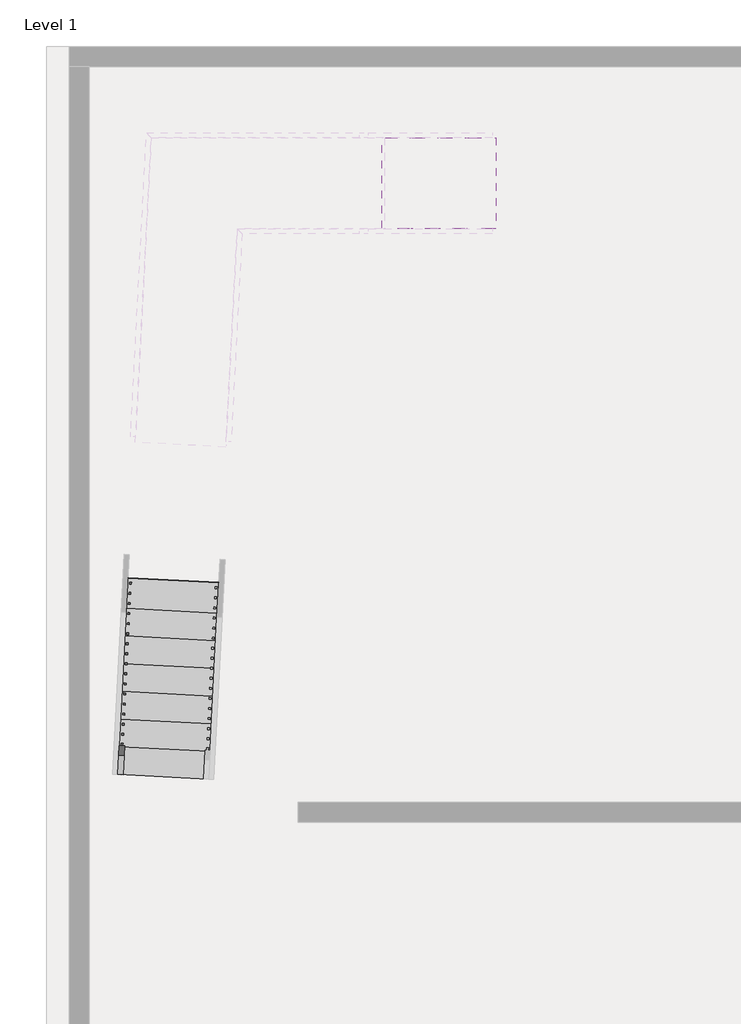
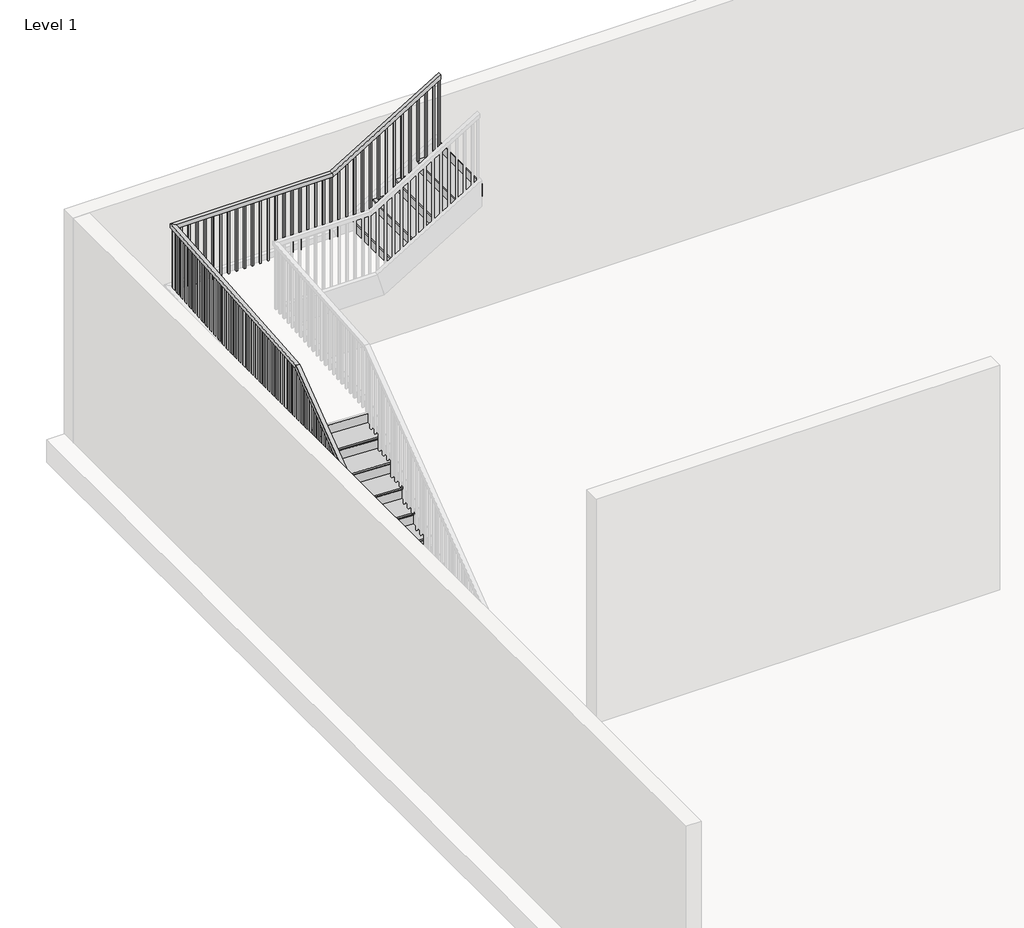
# One storey, part 2 of 3: 2 stair flights, 1 railing.
"""IFC4 building model written with IfcOpenShell, lengths in millimetres."""

from ifc_helpers import new_model, si_unit, frame, origin, place, context, project, spatial, polyline, outline, extrude, faceted_brep, transform, mapped, element, save
from components import stair_flight_fe3b1aa7, stair_flight_5ad97bb6

model = new_model("IFC4")

# Units and contexts
model_context = context("Model", 3, world=origin())
ifc_project = project(units=[si_unit("LENGTHUNIT", "METRE", prefix="MILLI")], contexts=[model_context])

# Site, building, storey
site = spatial("IfcSite", under=ifc_project)
building = spatial("IfcBuilding", under=site)
storey = spatial("IfcBuildingStorey", under=building, Name="Level 1", Elevation=0.0)

# Railing
placement = place(None, origin())
element("IfcRailing", 1, ObjectType="Handrail - Rectangular", at=placement, inside=storey, context=model_context, shape_type="SolidModel", body=[
    faceted_brep([(-19614.0949489, 10767.2493231, 1083.7333333), (-19614.0949489, 10767.2493231, 1024.3318731), (-19563.3645685, 10764.5906565, 1024.3318731), (-19563.3645685, 10764.5906565, 1083.7333333), (-19438.6229548, 14115.4544272, 3115.7333333), (-19437.8801815, 14129.6273865, 3064.9333333), (-19387.1498011, 14126.9687199, 3064.9333333), (-19387.8925745, 14112.7957607, 3115.7333333), (-19277.7278471, 17185.5159704, 3115.7333333), (-19277.7278471, 17185.5159704, 3064.9333333), (-19229.5204471, 17134.7159704, 3064.9333333), (-19229.5204471, 17134.7159704, 3115.7333333), (-17229.733929, 17185.5159704, 3115.7333333), (-17215.5415195, 17185.5159704, 3064.9333333), (-17215.5415195, 17134.7159704, 3064.9333333), (-17229.733929, 17134.7159704, 3115.7333333), (-15832.733929, 17185.5159704, 3962.4), (-15832.733929, 17134.7159704, 3962.4), (-15832.733929, 17134.7159704, 3902.9985397), (-15832.733929, 17185.5159704, 3902.9985397)], [[[0, 1, 2, 3]], [[1, 0, 4, 5]], [[2, 1, 5, 6]], [[3, 2, 6, 7]], [[0, 3, 7, 4]], [[5, 4, 8, 9]], [[6, 5, 9, 10]], [[7, 6, 10, 11]], [[4, 7, 11, 8]], [[9, 8, 12, 13]], [[10, 9, 13, 14]], [[11, 10, 14, 15]], [[8, 11, 15, 12]], [[16, 17, 18, 19]], [[13, 12, 16, 19]], [[14, 13, 19, 18]], [[15, 14, 18, 17]], [[12, 15, 17, 16]]]),
    extrude(outline(polyline([(3851.0439943, -15918.458929), (2878.6666667, -15918.458929), (2878.6666667, -15899.408929), (3862.5894488, -15899.408929), (3851.0439943, -15918.458929)])), frame((0.0, 17150.5909704, 0.0), z_axis=(0.0, 1.0, 0.0), x_axis=(0.0, 0.0, 1.0)), (0.0, 0.0, 1.0), 19.05),
    extrude(outline(polyline([(3789.4682367, -16020.058929), (2878.6666667, -16020.058929), (2878.6666667, -16001.008929), (3801.0136913, -16001.008929), (3789.4682367, -16020.058929)])), frame((0.0, 17150.5909704, 0.0), z_axis=(0.0, 1.0, 0.0), x_axis=(0.0, 0.0, 1.0)), (0.0, 0.0, 1.0), 19.05),
    extrude(outline(polyline([(3727.8924791, -16121.658929), (2878.6666667, -16121.658929), (2878.6666667, -16102.608929), (3739.4379337, -16102.608929), (3727.8924791, -16121.658929)])), frame((0.0, 17150.5909704, 0.0), z_axis=(0.0, 1.0, 0.0), x_axis=(0.0, 0.0, 1.0)), (0.0, 0.0, 1.0), 19.05),
    extrude(outline(polyline([(3666.3167216, -16223.258929), (2709.3333333, -16223.258929), (2709.3333333, -16204.208929), (3677.8621761, -16204.208929), (3666.3167216, -16223.258929)])), frame((0.0, 17150.5909704, 0.0), z_axis=(0.0, 1.0, 0.0), x_axis=(0.0, 0.0, 1.0)), (0.0, 0.0, 1.0), 19.05),
    extrude(outline(polyline([(3604.740964, -16324.858929), (2709.3333333, -16324.858929), (2709.3333333, -16305.808929), (3616.2864185, -16305.808929), (3604.740964, -16324.858929)])), frame((0.0, 17150.5909704, 0.0), z_axis=(0.0, 1.0, 0.0), x_axis=(0.0, 0.0, 1.0)), (0.0, 0.0, 1.0), 19.05),
    extrude(outline(polyline([(3543.1652064, -16426.458929), (2540.0, -16426.458929), (2540.0, -16407.408929), (3554.710661, -16407.408929), (3543.1652064, -16426.458929)])), frame((0.0, 17150.5909704, 0.0), z_axis=(0.0, 1.0, 0.0), x_axis=(0.0, 0.0, 1.0)), (0.0, 0.0, 1.0), 19.05),
    extrude(outline(polyline([(3481.5894488, -16528.058929), (2540.0, -16528.058929), (2540.0, -16509.008929), (3493.1349034, -16509.008929), (3481.5894488, -16528.058929)])), frame((0.0, 17150.5909704, 0.0), z_axis=(0.0, 1.0, 0.0), x_axis=(0.0, 0.0, 1.0)), (0.0, 0.0, 1.0), 19.05),
    extrude(outline(polyline([(3420.0136913, -16629.658929), (2540.0, -16629.658929), (2540.0, -16610.608929), (3431.5591458, -16610.608929), (3420.0136913, -16629.658929)])), frame((0.0, 17150.5909704, 0.0), z_axis=(0.0, 1.0, 0.0), x_axis=(0.0, 0.0, 1.0)), (0.0, 0.0, 1.0), 19.05),
    extrude(outline(polyline([(3358.4379337, -16731.258929), (2370.6666667, -16731.258929), (2370.6666667, -16712.208929), (3369.9833882, -16712.208929), (3358.4379337, -16731.258929)])), frame((0.0, 17150.5909704, 0.0), z_axis=(0.0, 1.0, 0.0), x_axis=(0.0, 0.0, 1.0)), (0.0, 0.0, 1.0), 19.05),
    extrude(outline(polyline([(3296.8621761, -16832.858929), (2370.6666667, -16832.858929), (2370.6666667, -16813.808929), (3308.4076307, -16813.808929), (3296.8621761, -16832.858929)])), frame((0.0, 17150.5909704, 0.0), z_axis=(0.0, 1.0, 0.0), x_axis=(0.0, 0.0, 1.0)), (0.0, 0.0, 1.0), 19.05),
    extrude(outline(polyline([(3235.2864185, -16934.458929), (2370.6666667, -16934.458929), (2370.6666667, -16915.408929), (3246.8318731, -16915.408929), (3235.2864185, -16934.458929)])), frame((0.0, 17150.5909704, 0.0), z_axis=(0.0, 1.0, 0.0), x_axis=(0.0, 0.0, 1.0)), (0.0, 0.0, 1.0), 19.05),
    extrude(outline(polyline([(3173.710661, -17036.058929), (2201.3333333, -17036.058929), (2201.3333333, -17017.008929), (3185.2561155, -17017.008929), (3173.710661, -17036.058929)])), frame((0.0, 17150.5909704, 0.0), z_axis=(0.0, 1.0, 0.0), x_axis=(0.0, 0.0, 1.0)), (0.0, 0.0, 1.0), 19.05),
    extrude(outline(polyline([(3112.1349034, -17137.658929), (2201.3333333, -17137.658929), (2201.3333333, -17118.608929), (3123.6803579, -17118.608929), (3112.1349034, -17137.658929)])), frame((0.0, 17150.5909704, 0.0), z_axis=(0.0, 1.0, 0.0), x_axis=(0.0, 0.0, 1.0)), (0.0, 0.0, 1.0), 19.05),
    extrude(outline(polyline([(-17332.7491471, 17169.6409704), (-17313.6991471, 17169.6409704), (-17313.6991471, 17150.5909704), (-17332.7491471, 17150.5909704), (-17332.7491471, 17169.6409704)])), frame((0.0, 0.0, 2201.3333333), z_axis=(0.0, 0.0, 1.0), x_axis=(1.0, 0.0, 0.0)), (0.0, 0.0, 1.0), 863.6),
    extrude(outline(polyline([(-17434.3491471, 17169.6409704), (-17415.2991471, 17169.6409704), (-17415.2991471, 17150.5909704), (-17434.3491471, 17150.5909704), (-17434.3491471, 17169.6409704)])), frame((0.0, 0.0, 2201.3333333), z_axis=(0.0, 0.0, 1.0), x_axis=(1.0, 0.0, 0.0)), (0.0, 0.0, 1.0), 863.6),
    extrude(outline(polyline([(-17535.9491471, 17169.6409704), (-17516.8991471, 17169.6409704), (-17516.8991471, 17150.5909704), (-17535.9491471, 17150.5909704), (-17535.9491471, 17169.6409704)])), frame((0.0, 0.0, 2201.3333333), z_axis=(0.0, 0.0, 1.0), x_axis=(1.0, 0.0, 0.0)), (0.0, 0.0, 1.0), 863.6),
    extrude(outline(polyline([(-17637.5491471, 17169.6409704), (-17618.4991471, 17169.6409704), (-17618.4991471, 17150.5909704), (-17637.5491471, 17150.5909704), (-17637.5491471, 17169.6409704)])), frame((0.0, 0.0, 2201.3333333), z_axis=(0.0, 0.0, 1.0), x_axis=(1.0, 0.0, 0.0)), (0.0, 0.0, 1.0), 863.6),
    extrude(outline(polyline([(-17739.1491471, 17169.6409704), (-17720.0991471, 17169.6409704), (-17720.0991471, 17150.5909704), (-17739.1491471, 17150.5909704), (-17739.1491471, 17169.6409704)])), frame((0.0, 0.0, 2201.3333333), z_axis=(0.0, 0.0, 1.0), x_axis=(1.0, 0.0, 0.0)), (0.0, 0.0, 1.0), 863.6),
    extrude(outline(polyline([(-17840.7491471, 17169.6409704), (-17821.6991471, 17169.6409704), (-17821.6991471, 17150.5909704), (-17840.7491471, 17150.5909704), (-17840.7491471, 17169.6409704)])), frame((0.0, 0.0, 2201.3333333), z_axis=(0.0, 0.0, 1.0), x_axis=(1.0, 0.0, 0.0)), (0.0, 0.0, 1.0), 863.6),
    extrude(outline(polyline([(-17942.3491471, 17169.6409704), (-17923.2991471, 17169.6409704), (-17923.2991471, 17150.5909704), (-17942.3491471, 17150.5909704), (-17942.3491471, 17169.6409704)])), frame((0.0, 0.0, 2201.3333333), z_axis=(0.0, 0.0, 1.0), x_axis=(1.0, 0.0, 0.0)), (0.0, 0.0, 1.0), 863.6),
    extrude(outline(polyline([(-18043.9491471, 17169.6409704), (-18024.8991471, 17169.6409704), (-18024.8991471, 17150.5909704), (-18043.9491471, 17150.5909704), (-18043.9491471, 17169.6409704)])), frame((0.0, 0.0, 2201.3333333), z_axis=(0.0, 0.0, 1.0), x_axis=(1.0, 0.0, 0.0)), (0.0, 0.0, 1.0), 863.6),
    extrude(outline(polyline([(-18145.5491471, 17169.6409704), (-18126.4991471, 17169.6409704), (-18126.4991471, 17150.5909704), (-18145.5491471, 17150.5909704), (-18145.5491471, 17169.6409704)])), frame((0.0, 0.0, 2201.3333333), z_axis=(0.0, 0.0, 1.0), x_axis=(1.0, 0.0, 0.0)), (0.0, 0.0, 1.0), 863.6),
    extrude(outline(polyline([(-18247.1491471, 17169.6409704), (-18228.0991471, 17169.6409704), (-18228.0991471, 17150.5909704), (-18247.1491471, 17150.5909704), (-18247.1491471, 17169.6409704)])), frame((0.0, 0.0, 2201.3333333), z_axis=(0.0, 0.0, 1.0), x_axis=(1.0, 0.0, 0.0)), (0.0, 0.0, 1.0), 863.6),
    extrude(outline(polyline([(-18348.7491471, 17169.6409704), (-18329.6991471, 17169.6409704), (-18329.6991471, 17150.5909704), (-18348.7491471, 17150.5909704), (-18348.7491471, 17169.6409704)])), frame((0.0, 0.0, 2201.3333333), z_axis=(0.0, 0.0, 1.0), x_axis=(1.0, 0.0, 0.0)), (0.0, 0.0, 1.0), 863.6),
    extrude(outline(polyline([(-18450.3491471, 17169.6409704), (-18431.2991471, 17169.6409704), (-18431.2991471, 17150.5909704), (-18450.3491471, 17150.5909704), (-18450.3491471, 17169.6409704)])), frame((0.0, 0.0, 2201.3333333), z_axis=(0.0, 0.0, 1.0), x_axis=(1.0, 0.0, 0.0)), (0.0, 0.0, 1.0), 863.6),
    extrude(outline(polyline([(-18551.9491471, 17169.6409704), (-18532.8991471, 17169.6409704), (-18532.8991471, 17150.5909704), (-18551.9491471, 17150.5909704), (-18551.9491471, 17169.6409704)])), frame((0.0, 0.0, 2201.3333333), z_axis=(0.0, 0.0, 1.0), x_axis=(1.0, 0.0, 0.0)), (0.0, 0.0, 1.0), 863.6),
    extrude(outline(polyline([(-18653.5491471, 17169.6409704), (-18634.4991471, 17169.6409704), (-18634.4991471, 17150.5909704), (-18653.5491471, 17150.5909704), (-18653.5491471, 17169.6409704)])), frame((0.0, 0.0, 2201.3333333), z_axis=(0.0, 0.0, 1.0), x_axis=(1.0, 0.0, 0.0)), (0.0, 0.0, 1.0), 863.6),
    extrude(outline(polyline([(-18755.1491471, 17169.6409704), (-18736.0991471, 17169.6409704), (-18736.0991471, 17150.5909704), (-18755.1491471, 17150.5909704), (-18755.1491471, 17169.6409704)])), frame((0.0, 0.0, 2201.3333333), z_axis=(0.0, 0.0, 1.0), x_axis=(1.0, 0.0, 0.0)), (0.0, 0.0, 1.0), 863.6),
    extrude(outline(polyline([(-18856.7491471, 17169.6409704), (-18837.6991471, 17169.6409704), (-18837.6991471, 17150.5909704), (-18856.7491471, 17150.5909704), (-18856.7491471, 17169.6409704)])), frame((0.0, 0.0, 2201.3333333), z_axis=(0.0, 0.0, 1.0), x_axis=(1.0, 0.0, 0.0)), (0.0, 0.0, 1.0), 863.6),
    extrude(outline(polyline([(-18958.3491471, 17169.6409704), (-18939.2991471, 17169.6409704), (-18939.2991471, 17150.5909704), (-18958.3491471, 17150.5909704), (-18958.3491471, 17169.6409704)])), frame((0.0, 0.0, 2201.3333333), z_axis=(0.0, 0.0, 1.0), x_axis=(1.0, 0.0, 0.0)), (0.0, 0.0, 1.0), 863.6),
    extrude(outline(polyline([(-19059.9491471, 17169.6409704), (-19040.8991471, 17169.6409704), (-19040.8991471, 17150.5909704), (-19059.9491471, 17150.5909704), (-19059.9491471, 17169.6409704)])), frame((0.0, 0.0, 2201.3333333), z_axis=(0.0, 0.0, 1.0), x_axis=(1.0, 0.0, 0.0)), (0.0, 0.0, 1.0), 863.6),
    extrude(outline(polyline([(-19161.5491471, 17169.6409704), (-19142.4991471, 17169.6409704), (-19142.4991471, 17150.5909704), (-19161.5491471, 17150.5909704), (-19161.5491471, 17169.6409704)])), frame((0.0, 0.0, 2201.3333333), z_axis=(0.0, 0.0, 1.0), x_axis=(1.0, 0.0, 0.0)), (0.0, 0.0, 1.0), 863.6),
    extrude(outline(polyline([(-19263.7482163, 17148.9344695), (-19262.7512163, 17167.9583622), (-19243.7273237, 17166.9613622), (-19244.7243237, 17147.9374696), (-19263.7482163, 17148.9344695)])), frame((0.0, 0.0, 2201.3333333), z_axis=(0.0, 0.0, 1.0), x_axis=(1.0, 0.0, 0.0)), (0.0, 0.0, 1.0), 863.6),
    extrude(outline(polyline([(-19269.0655495, 17047.4737088), (-19268.0685495, 17066.4976015), (-19249.0446569, 17065.5006015), (-19250.0416568, 17046.4767089), (-19269.0655495, 17047.4737088)])), frame((0.0, 0.0, 2201.3333333), z_axis=(0.0, 0.0, 1.0), x_axis=(1.0, 0.0, 0.0)), (0.0, 0.0, 1.0), 863.6),
    extrude(outline(polyline([(-19274.3828826, 16946.0129481), (-19273.3858826, 16965.0368407), (-19254.36199, 16964.0398408), (-19255.35899, 16945.0159481), (-19274.3828826, 16946.0129481)])), frame((0.0, 0.0, 2201.3333333), z_axis=(0.0, 0.0, 1.0), x_axis=(1.0, 0.0, 0.0)), (0.0, 0.0, 1.0), 863.6),
    extrude(outline(polyline([(-19279.7002158, 16844.5521874), (-19278.7032158, 16863.57608), (-19259.6793232, 16862.57908), (-19260.6763231, 16843.5551874), (-19279.7002158, 16844.5521874)])), frame((0.0, 0.0, 2201.3333333), z_axis=(0.0, 0.0, 1.0), x_axis=(1.0, 0.0, 0.0)), (0.0, 0.0, 1.0), 863.6),
    extrude(outline(polyline([(-19285.0175489, 16743.0914266), (-19284.020549, 16762.1153193), (-19264.9966563, 16761.1183193), (-19265.9936563, 16742.0944267), (-19285.0175489, 16743.0914266)])), frame((0.0, 0.0, 2201.3333333), z_axis=(0.0, 0.0, 1.0), x_axis=(1.0, 0.0, 0.0)), (0.0, 0.0, 1.0), 863.6),
    extrude(outline(polyline([(-19290.3348821, 16641.6306659), (-19289.3378821, 16660.6545585), (-19270.3139895, 16659.6575586), (-19271.3109894, 16640.6336659), (-19290.3348821, 16641.6306659)])), frame((0.0, 0.0, 2201.3333333), z_axis=(0.0, 0.0, 1.0), x_axis=(1.0, 0.0, 0.0)), (0.0, 0.0, 1.0), 863.6),
    extrude(outline(polyline([(-19295.6522152, 16540.1699052), (-19294.6552153, 16559.1937978), (-19275.6313226, 16558.1967978), (-19276.6283226, 16539.1729052), (-19295.6522152, 16540.1699052)])), frame((0.0, 0.0, 2201.3333333), z_axis=(0.0, 0.0, 1.0), x_axis=(1.0, 0.0, 0.0)), (0.0, 0.0, 1.0), 863.6),
    extrude(outline(polyline([(-19300.9695484, 16438.7091444), (-19299.9725484, 16457.7330371), (-19280.9486558, 16456.7360371), (-19281.9456557, 16437.7121445), (-19300.9695484, 16438.7091444)])), frame((0.0, 0.0, 2201.3333333), z_axis=(0.0, 0.0, 1.0), x_axis=(1.0, 0.0, 0.0)), (0.0, 0.0, 1.0), 863.6),
    extrude(outline(polyline([(-19306.2868815, 16337.2483837), (-19305.2898816, 16356.2722763), (-19286.2659889, 16355.2752764), (-19287.2629889, 16336.2513837), (-19306.2868815, 16337.2483837)])), frame((0.0, 0.0, 2201.3333333), z_axis=(0.0, 0.0, 1.0), x_axis=(1.0, 0.0, 0.0)), (0.0, 0.0, 1.0), 863.6),
    extrude(outline(polyline([(-19311.6042147, 16235.787623), (-19310.6072147, 16254.8115156), (-19291.5833221, 16253.8145156), (-19292.5803221, 16234.790623), (-19311.6042147, 16235.787623)])), frame((0.0, 0.0, 2201.3333333), z_axis=(0.0, 0.0, 1.0), x_axis=(1.0, 0.0, 0.0)), (0.0, 0.0, 1.0), 863.6),
    extrude(outline(polyline([(-19316.9215478, 16134.3268622), (-19315.9245479, 16153.3507549), (-19296.9006552, 16152.3537549), (-19297.8976552, 16133.3298623), (-19316.9215478, 16134.3268622)])), frame((0.0, 0.0, 2201.3333333), z_axis=(0.0, 0.0, 1.0), x_axis=(1.0, 0.0, 0.0)), (0.0, 0.0, 1.0), 863.6),
    extrude(outline(polyline([(-19322.238881, 16032.8661015), (-19321.241881, 16051.8899941), (-19302.2179884, 16050.8929942), (-19303.2149884, 16031.8691015), (-19322.238881, 16032.8661015)])), frame((0.0, 0.0, 2201.3333333), z_axis=(0.0, 0.0, 1.0), x_axis=(1.0, 0.0, 0.0)), (0.0, 0.0, 1.0), 863.6),
    extrude(outline(polyline([(-19327.5562142, 15931.4053408), (-19326.5592142, 15950.4292334), (-19307.5353216, 15949.4322334), (-19308.5323215, 15930.4083408), (-19327.5562142, 15931.4053408)])), frame((0.0, 0.0, 2201.3333333), z_axis=(0.0, 0.0, 1.0), x_axis=(1.0, 0.0, 0.0)), (0.0, 0.0, 1.0), 863.6),
    extrude(outline(polyline([(-19332.8735473, 15829.94458), (-19331.8765473, 15848.9684727), (-19312.8526547, 15847.9714727), (-19313.8496547, 15828.9475801), (-19332.8735473, 15829.94458)])), frame((0.0, 0.0, 2201.3333333), z_axis=(0.0, 0.0, 1.0), x_axis=(1.0, 0.0, 0.0)), (0.0, 0.0, 1.0), 863.6),
    extrude(outline(polyline([(-19338.1908805, 15728.4838193), (-19337.1938805, 15747.507712), (-19318.1699879, 15746.510712), (-19319.1669878, 15727.4868193), (-19338.1908805, 15728.4838193)])), frame((0.0, 0.0, 2201.3333333), z_axis=(0.0, 0.0, 1.0), x_axis=(1.0, 0.0, 0.0)), (0.0, 0.0, 1.0), 863.6),
    extrude(outline(polyline([(-19343.5082136, 15627.0230586), (-19342.5112137, 15646.0469512), (-19323.487321, 15645.0499513), (-19324.484321, 15626.0260586), (-19343.5082136, 15627.0230586)])), frame((0.0, 0.0, 2201.3333333), z_axis=(0.0, 0.0, 1.0), x_axis=(1.0, 0.0, 0.0)), (0.0, 0.0, 1.0), 863.6),
    extrude(outline(polyline([(-19348.8255468, 15525.5622979), (-19347.8285468, 15544.5861905), (-19328.8046542, 15543.5891905), (-19329.8016541, 15524.5652979), (-19348.8255468, 15525.5622979)])), frame((0.0, 0.0, 2201.3333333), z_axis=(0.0, 0.0, 1.0), x_axis=(1.0, 0.0, 0.0)), (0.0, 0.0, 1.0), 863.6),
    extrude(outline(polyline([(-19354.1428799, 15424.1015371), (-19353.14588, 15443.1254298), (-19334.1219873, 15442.1284298), (-19335.1189873, 15423.1045372), (-19354.1428799, 15424.1015371)])), frame((0.0, 0.0, 2201.3333333), z_axis=(0.0, 0.0, 1.0), x_axis=(1.0, 0.0, 0.0)), (0.0, 0.0, 1.0), 863.6),
    extrude(outline(polyline([(-19359.4602131, 15322.6407764), (-19358.4632131, 15341.664669), (-19339.4393205, 15340.6676691), (-19340.4363204, 15321.6437764), (-19359.4602131, 15322.6407764)])), frame((0.0, 0.0, 2201.3333333), z_axis=(0.0, 0.0, 1.0), x_axis=(1.0, 0.0, 0.0)), (0.0, 0.0, 1.0), 863.6),
    extrude(outline(polyline([(-19364.7775462, 15221.1800157), (-19363.7805463, 15240.2039083), (-19344.7566536, 15239.2069083), (-19345.7536536, 15220.1830157), (-19364.7775462, 15221.1800157)])), frame((0.0, 0.0, 2201.3333333), z_axis=(0.0, 0.0, 1.0), x_axis=(1.0, 0.0, 0.0)), (0.0, 0.0, 1.0), 863.6),
    extrude(outline(polyline([(-19370.0948794, 15119.7192549), (-19369.0978794, 15138.7431476), (-19350.0739868, 15137.7461476), (-19351.0709868, 15118.722255), (-19370.0948794, 15119.7192549)])), frame((0.0, 0.0, 2201.3333333), z_axis=(0.0, 0.0, 1.0), x_axis=(1.0, 0.0, 0.0)), (0.0, 0.0, 1.0), 863.6),
    extrude(outline(polyline([(-19375.4122125, 15018.2584942), (-19374.4152126, 15037.2823868), (-19355.3913199, 15036.2853869), (-19356.3883199, 15017.2614942), (-19375.4122125, 15018.2584942)])), frame((0.0, 0.0, 2201.3333333), z_axis=(0.0, 0.0, 1.0), x_axis=(1.0, 0.0, 0.0)), (0.0, 0.0, 1.0), 863.6),
    extrude(outline(polyline([(-19380.7295457, 14916.7977335), (-19379.7325457, 14935.8216261), (-19360.7086531, 14934.8246261), (-19361.7056531, 14915.8007335), (-19380.7295457, 14916.7977335)])), frame((0.0, 0.0, 2201.3333333), z_axis=(0.0, 0.0, 1.0), x_axis=(1.0, 0.0, 0.0)), (0.0, 0.0, 1.0), 863.6),
    extrude(outline(polyline([(-19386.0468789, 14815.3369727), (-19385.0498789, 14834.3608654), (-19366.0259863, 14833.3638654), (-19367.0229862, 14814.3399728), (-19386.0468789, 14815.3369727)])), frame((0.0, 0.0, 2201.3333333), z_axis=(0.0, 0.0, 1.0), x_axis=(1.0, 0.0, 0.0)), (0.0, 0.0, 1.0), 863.6),
    extrude(outline(polyline([(-19391.364212, 14713.876212), (-19390.367212, 14732.9001046), (-19371.3433194, 14731.9031047), (-19372.3403194, 14712.879212), (-19391.364212, 14713.876212)])), frame((0.0, 0.0, 2201.3333333), z_axis=(0.0, 0.0, 1.0), x_axis=(1.0, 0.0, 0.0)), (0.0, 0.0, 1.0), 863.6),
    extrude(outline(polyline([(-19396.6815452, 14612.4154513), (-19395.6845452, 14631.4393439), (-19376.6606526, 14630.4423439), (-19377.6576525, 14611.4184513), (-19396.6815452, 14612.4154513)])), frame((0.0, 0.0, 2201.3333333), z_axis=(0.0, 0.0, 1.0), x_axis=(1.0, 0.0, 0.0)), (0.0, 0.0, 1.0), 863.6),
    extrude(outline(polyline([(-19401.9988783, 14510.9546905), (-19401.0018784, 14529.9785832), (-19381.9779857, 14528.9815832), (-19382.9749857, 14509.9576906), (-19401.9988783, 14510.9546905)])), frame((0.0, 0.0, 2201.3333333), z_axis=(0.0, 0.0, 1.0), x_axis=(1.0, 0.0, 0.0)), (0.0, 0.0, 1.0), 863.6),
    extrude(outline(polyline([(-19407.3162115, 14409.4939298), (-19406.3192115, 14428.5178224), (-19387.2953189, 14427.5208225), (-19388.2923188, 14408.4969298), (-19407.3162115, 14409.4939298)])), frame((0.0, 0.0, 2201.3333333), z_axis=(0.0, 0.0, 1.0), x_axis=(1.0, 0.0, 0.0)), (0.0, 0.0, 1.0), 863.6),
    extrude(outline(polyline([(-19412.6335446, 14308.0331691), (-19411.6365447, 14327.0570617), (-19392.612652, 14326.0600617), (-19393.609652, 14307.0361691), (-19412.6335446, 14308.0331691)])), frame((0.0, 0.0, 2201.3333333), z_axis=(0.0, 0.0, 1.0), x_axis=(1.0, 0.0, 0.0)), (0.0, 0.0, 1.0), 863.6),
    extrude(outline(polyline([(-19417.9508778, 14206.5724083), (-19416.9538778, 14225.596301), (-19397.9299852, 14224.599301), (-19398.9269851, 14205.5754084), (-19417.9508778, 14206.5724083)])), frame((0.0, 0.0, 2201.3333333), z_axis=(0.0, 0.0, 1.0), x_axis=(1.0, 0.0, 0.0)), (0.0, 0.0, 1.0), 863.6),
    extrude(outline(polyline([(234.3727273, 19.0500001), (1191.3561155, 19.0500001), (1191.3561155, 0.0), (222.8272727, 0.0), (234.3727273, 19.0500001)])), frame((-19408.5646515, 14021.6777796, 3223.3561155), z_axis=(-0.9986295347545738, 0.052335956242945125, 0.0), x_axis=(0.0, 0.0, -1.0)), (0.0, 0.0, 1.0), 19.05),
    extrude(outline(polyline([(234.3727272, 19.05), (1129.7803579, 19.05), (1129.7803579, 0.0), (222.8272727, 0.0), (234.3727272, 19.05)])), frame((-19413.8819846, 13920.2170188, 3161.7803579), z_axis=(-0.9986295347545738, 0.052335956242945125, 0.0), x_axis=(0.0, 0.0, -1.0)), (0.0, 0.0, 1.0), 19.05),
    extrude(outline(polyline([(234.3727273, 19.05), (1237.5379337, 19.05), (1237.5379337, 0.0), (222.8272728, 0.0), (234.3727273, 19.05)])), frame((-19419.1993178, 13818.7562581, 3100.2046004), z_axis=(-0.9986295347545738, 0.052335956242945125, 0.0), x_axis=(0.0, 0.0, -1.0)), (0.0, 0.0, 1.0), 19.05),
    extrude(outline(polyline([(234.3727273, 19.0500001), (1175.9621761, 19.0500001), (1175.9621761, 0.0), (222.8272728, 0.0), (234.3727273, 19.0500001)])), frame((-19424.5166509, 13717.2954974, 3038.6288428), z_axis=(-0.9986295347545738, 0.052335956242945125, 0.0), x_axis=(0.0, 0.0, -1.0)), (0.0, 0.0, 1.0), 19.05),
    extrude(outline(polyline([(234.3727273, 19.05), (1114.3864185, 19.05), (1114.3864185, 0.0), (222.8272727, 0.0), (234.3727273, 19.05)])), frame((-19429.8339841, 13615.8347366, 2977.0530852), z_axis=(-0.9986295347545738, 0.052335956242945125, 0.0), x_axis=(0.0, 0.0, -1.0)), (0.0, 0.0, 1.0), 19.05),
    extrude(outline(polyline([(234.3727272, 19.05), (1222.1439943, 19.05), (1222.1439943, 0.0), (222.8272727, 0.0), (234.3727272, 19.05)])), frame((-19435.1513173, 13514.3739759, 2915.4773276), z_axis=(-0.9986295347545738, 0.052335956242945125, 0.0), x_axis=(0.0, 0.0, -1.0)), (0.0, 0.0, 1.0), 19.05),
    extrude(outline(polyline([(234.3727272, 19.0500001), (1160.5682367, 19.0500001), (1160.5682367, 0.0), (222.8272727, 0.0), (234.3727272, 19.0500001)])), frame((-19440.4686504, 13412.9132152, 2853.90157), z_axis=(-0.9986295347545738, 0.052335956242945125, 0.0), x_axis=(0.0, 0.0, -1.0)), (0.0, 0.0, 1.0), 19.05),
    extrude(outline(polyline([(234.3727273, 19.05), (1098.9924792, 19.05), (1098.9924792, 0.0), (222.8272728, 0.0), (234.3727273, 19.05)])), frame((-19445.7859836, 13311.4524544, 2792.3258125), z_axis=(-0.9986295347545738, 0.052335956242945125, 0.0), x_axis=(0.0, 0.0, -1.0)), (0.0, 0.0, 1.0), 19.05),
    extrude(outline(polyline([(234.3727273, 19.05), (1206.7500549, 19.05), (1206.7500549, 0.0), (222.8272727, 0.0), (234.3727273, 19.05)])), frame((-19451.1033167, 13209.9916937, 2730.7500549), z_axis=(-0.9986295347545738, 0.052335956242945125, 0.0), x_axis=(0.0, 0.0, -1.0)), (0.0, 0.0, 1.0), 19.05),
    extrude(outline(polyline([(234.3727273, 19.0500001), (1145.1742973, 19.0500001), (1145.1742973, 0.0), (222.8272727, 0.0), (234.3727273, 19.0500001)])), frame((-19456.4206499, 13108.530933, 2669.1742973), z_axis=(-0.9986295347545738, 0.052335956242945125, 0.0), x_axis=(0.0, 0.0, -1.0)), (0.0, 0.0, 1.0), 19.05),
    extrude(outline(polyline([(234.3727272, 19.05), (1083.5985397, 19.05), (1083.5985397, 0.0), (222.8272727, 0.0), (234.3727272, 19.05)])), frame((-19461.737983, 13007.0701722, 2607.5985397), z_axis=(-0.9986295347545738, 0.052335956242945125, 0.0), x_axis=(0.0, 0.0, -1.0)), (0.0, 0.0, 1.0), 19.05),
    extrude(outline(polyline([(234.3727273, 19.05), (1191.3561155, 19.05), (1191.3561155, 0.0), (222.8272728, 0.0), (234.3727273, 19.05)])), frame((-19467.0553162, 12905.6094115, 2546.0227822), z_axis=(-0.9986295347545738, 0.052335956242945125, 0.0), x_axis=(0.0, 0.0, -1.0)), (0.0, 0.0, 1.0), 19.05),
    extrude(outline(polyline([(234.3727273, 19.0500001), (1129.7803579, 19.0500001), (1129.7803579, 0.0), (222.8272727, 0.0), (234.3727273, 19.0500001)])), frame((-19472.3726493, 12804.1486508, 2484.4470246), z_axis=(-0.9986295347545738, 0.052335956242945125, 0.0), x_axis=(0.0, 0.0, -1.0)), (0.0, 0.0, 1.0), 19.05),
    extrude(outline(polyline([(234.3727273, 19.0500001), (1237.5379337, 19.0500001), (1237.5379337, 0.0), (222.8272727, 0.0), (234.3727273, 19.0500001)])), frame((-19477.6899825, 12702.6878901, 2422.871267), z_axis=(-0.9986295347545738, 0.052335956242945125, 0.0), x_axis=(0.0, 0.0, -1.0)), (0.0, 0.0, 1.0), 19.05),
    extrude(outline(polyline([(234.3727272, 19.05), (1175.9621761, 19.05), (1175.9621761, 0.0), (222.8272727, 0.0), (234.3727272, 19.05)])), frame((-19483.0073156, 12601.2271293, 2361.2955094), z_axis=(-0.9986295347545738, 0.052335956242945125, 0.0), x_axis=(0.0, 0.0, -1.0)), (0.0, 0.0, 1.0), 19.05),
    extrude(outline(polyline([(234.3727273, 19.05), (1114.3864186, 19.05), (1114.3864186, 0.0), (222.8272728, 0.0), (234.3727273, 19.05)])), frame((-19488.3246488, 12499.7663686, 2299.7197519), z_axis=(-0.9986295347545738, 0.052335956242945125, 0.0), x_axis=(0.0, 0.0, -1.0)), (0.0, 0.0, 1.0), 19.05),
    extrude(outline(polyline([(234.3727273, 19.0500001), (1222.1439943, 19.0500001), (1222.1439943, 0.0), (222.8272727, 0.0), (234.3727273, 19.0500001)])), frame((-19493.641982, 12398.3056079, 2238.1439943), z_axis=(-0.9986295347545738, 0.052335956242945125, 0.0), x_axis=(0.0, 0.0, -1.0)), (0.0, 0.0, 1.0), 19.05),
    extrude(outline(polyline([(234.3727273, 19.05), (1160.5682367, 19.05), (1160.5682367, 0.0), (222.8272727, 0.0), (234.3727273, 19.05)])), frame((-19498.9593151, 12296.8448471, 2176.5682367), z_axis=(-0.9986295347545738, 0.052335956242945125, 0.0), x_axis=(0.0, 0.0, -1.0)), (0.0, 0.0, 1.0), 19.05),
    extrude(outline(polyline([(234.3727272, 19.05), (1098.9924791, 19.05), (1098.9924791, 0.0), (222.8272727, 0.0), (234.3727272, 19.05)])), frame((-19504.2766483, 12195.3840864, 2114.9924791), z_axis=(-0.9986295347545738, 0.052335956242945125, 0.0), x_axis=(0.0, 0.0, -1.0)), (0.0, 0.0, 1.0), 19.05),
    extrude(outline(polyline([(234.3727273, 19.0500001), (1206.7500549, 19.0500001), (1206.7500549, 0.0), (222.8272728, 0.0), (234.3727273, 19.0500001)])), frame((-19509.5939814, 12093.9233257, 2053.4167216), z_axis=(-0.9986295347545738, 0.052335956242945125, 0.0), x_axis=(0.0, 0.0, -1.0)), (0.0, 0.0, 1.0), 19.05),
    extrude(outline(polyline([(234.3727273, 19.05), (1145.1742973, 19.05), (1145.1742973, 0.0), (222.8272727, 0.0), (234.3727273, 19.05)])), frame((-19514.9113146, 11992.4625649, 1991.840964), z_axis=(-0.9986295347545738, 0.052335956242945125, 0.0), x_axis=(0.0, 0.0, -1.0)), (0.0, 0.0, 1.0), 19.05),
    extrude(outline(polyline([(234.3727273, 19.05), (1083.5985397, 19.05), (1083.5985397, 0.0), (222.8272727, 0.0), (234.3727273, 19.05)])), frame((-19520.2286477, 11891.0018042, 1930.2652064), z_axis=(-0.9986295347545738, 0.052335956242945125, 0.0), x_axis=(0.0, 0.0, -1.0)), (0.0, 0.0, 1.0), 19.05),
    extrude(outline(polyline([(234.3727272, 19.0500001), (1191.3561155, 19.0500001), (1191.3561155, 0.0), (222.8272727, 0.0), (234.3727272, 19.0500001)])), frame((-19525.5459809, 11789.5410435, 1868.6894488), z_axis=(-0.9986295347545738, 0.052335956242945125, 0.0), x_axis=(0.0, 0.0, -1.0)), (0.0, 0.0, 1.0), 19.05),
    extrude(outline(polyline([(234.3727273, 19.05), (1129.780358, 19.05), (1129.780358, 0.0), (222.8272728, 0.0), (234.3727273, 19.05)])), frame((-19530.863314, 11688.0802827, 1807.1136913), z_axis=(-0.9986295347545738, 0.052335956242945125, 0.0), x_axis=(0.0, 0.0, -1.0)), (0.0, 0.0, 1.0), 19.05),
    extrude(outline(polyline([(234.3727273, 19.05), (1237.5379337, 19.05), (1237.5379337, 0.0), (222.8272727, 0.0), (234.3727273, 19.05)])), frame((-19536.1806472, 11586.619522, 1745.5379337), z_axis=(-0.9986295347545738, 0.052335956242945125, 0.0), x_axis=(0.0, 0.0, -1.0)), (0.0, 0.0, 1.0), 19.05),
    extrude(outline(polyline([(234.3727273, 19.0500001), (1175.9621761, 19.0500001), (1175.9621761, 0.0), (222.8272727, 0.0), (234.3727273, 19.0500001)])), frame((-19541.4979803, 11485.1587613, 1683.9621761), z_axis=(-0.9986295347545738, 0.052335956242945125, 0.0), x_axis=(0.0, 0.0, -1.0)), (0.0, 0.0, 1.0), 19.05),
    extrude(outline(polyline([(234.3727272, 19.05), (1114.3864185, 19.05), (1114.3864185, 0.0), (222.8272727, 0.0), (234.3727272, 19.05)])), frame((-19546.8153135, 11383.6980005, 1622.3864185), z_axis=(-0.9986295347545738, 0.052335956242945125, 0.0), x_axis=(0.0, 0.0, -1.0)), (0.0, 0.0, 1.0), 19.05),
    extrude(outline(polyline([(234.3727273, 19.05), (1222.1439943, 19.05), (1222.1439943, 0.0), (222.8272728, 0.0), (234.3727273, 19.05)])), frame((-19552.1326467, 11282.2372398, 1560.810661), z_axis=(-0.9986295347545738, 0.052335956242945125, 0.0), x_axis=(0.0, 0.0, -1.0)), (0.0, 0.0, 1.0), 19.05),
    extrude(outline(polyline([(234.3727273, 19.0500001), (1160.5682367, 19.0500001), (1160.5682367, 0.0), (222.8272727, 0.0), (234.3727273, 19.0500001)])), frame((-19557.4499798, 11180.7764791, 1499.2349034), z_axis=(-0.9986295347545738, 0.052335956242945125, 0.0), x_axis=(0.0, 0.0, -1.0)), (0.0, 0.0, 1.0), 19.05),
    extrude(outline(polyline([(234.3727273, 19.0500001), (1098.9924791, 19.0500001), (1098.9924791, 0.0), (222.8272727, 0.0), (234.3727273, 19.0500001)])), frame((-19562.767313, 11079.3157184, 1437.6591458), z_axis=(-0.9986295347545738, 0.052335956242945125, 0.0), x_axis=(0.0, 0.0, -1.0)), (0.0, 0.0, 1.0), 19.05),
    extrude(outline(polyline([(234.3727272, 19.05), (1206.7500549, 19.05), (1206.7500549, 0.0), (222.8272727, 0.0), (234.3727272, 19.05)])), frame((-19568.0846461, 10977.8549576, 1376.0833882), z_axis=(-0.9986295347545738, 0.052335956242945125, 0.0), x_axis=(0.0, 0.0, -1.0)), (0.0, 0.0, 1.0), 19.05),
    extrude(outline(polyline([(234.3727273, 19.05), (1145.1742974, 19.05), (1145.1742974, 0.0), (222.8272728, 0.0), (234.3727273, 19.05)])), frame((-19573.4019793, 10876.3941969, 1314.5076307), z_axis=(-0.9986295347545738, 0.052335956242945125, 0.0), x_axis=(0.0, 0.0, -1.0)), (0.0, 0.0, 1.0), 19.05),
    extrude(outline(polyline([(3050.5591458, -17239.258929), (2201.3333333, -17239.258929), (2201.3333333, -17220.208929), (3062.1046004, -17220.208929), (3050.5591458, -17239.258929)])), frame((0.0, 17150.5909704, 0.0), z_axis=(0.0, 1.0, 0.0), x_axis=(0.0, 0.0, 1.0)), (0.0, 0.0, 1.0), 19.05),
    extrude(outline(polyline([(-19263.6345934, 17151.102524), (-19262.6375934, 17170.1264167), (-19243.6137008, 17169.1294167), (-19244.6107007, 17150.105524), (-19263.6345934, 17151.102524)])), frame((0.0, 0.0, 2201.3333333), z_axis=(0.0, 0.0, 1.0), x_axis=(1.0, 0.0, 0.0)), (0.0, 0.0, 1.0), 863.6),
    extrude(outline(polyline([(-19423.2682109, 14105.1116476), (-19422.271211, 14124.1355403), (-19403.2473183, 14123.1385403), (-19404.2443183, 14104.1146476), (-19423.2682109, 14105.1116476)])), frame((0.0, 0.0, 2201.3333333), z_axis=(0.0, 0.0, 1.0), x_axis=(1.0, 0.0, 0.0)), (0.0, 0.0, 1.0), 863.6),
    extrude(outline(polyline([(3891.4530852, -15851.783929), (2878.6666667, -15851.783929), (2878.6666667, -15832.733929), (3902.9985397, -15832.733929), (3891.4530852, -15851.783929)])), frame((0.0, 17150.5909704, 0.0), z_axis=(0.0, 1.0, 0.0), x_axis=(0.0, 0.0, 1.0)), (0.0, 0.0, 1.0), 19.05),
    extrude(outline(polyline([(234.3727273, 19.0500001), (1089.3712671, 19.0500001), (1089.3712671, 0.0), (222.8272728, 0.0), (234.3727273, 19.0500001)])), frame((-19578.2208124, 10784.4453825, 1258.7046004), z_axis=(-0.9986295347545738, 0.052335956242945125, 0.0), x_axis=(0.0, 0.0, -1.0)), (0.0, 0.0, 1.0), 19.05),
])

# Stair flights
stair_flight_shape = stair_flight_fe3b1aa7(model_context)
element("IfcStairFlight", 2, ObjectType="2\" Tread 1\" Nosing 1/4\" Riser", at=placement, inside=storey, context=model_context, shape_type="MappedRepresentation", body=[
    mapped(stair_flight_shape, transform((0.0, 0.0, 0.0), x_axis=(1.0, 0.0, 0.0), y_axis=(0.0, 1.0, 0.0), z_axis=(0.0, 0.0, 1.0))),
])
stair_flight_2_shape = stair_flight_5ad97bb6(model_context)
element("IfcStairFlight", 3, ObjectType="2\" Tread 1\" Nosing 1/4\" Riser", at=placement, inside=storey, context=model_context, shape_type="MappedRepresentation", body=[
    mapped(stair_flight_2_shape, transform((0.0, 0.0, 0.0), x_axis=(1.0, 0.0, 0.0), y_axis=(0.0, 1.0, 0.0), z_axis=(0.0, 0.0, 1.0))),
])

save(model, "model.ifc")

# Revit data of these elements
# Type "Handrail - Rectangular"
#   Assembly Code = "C2010400"
#   built-in parameter 1008612 = 0.0416667 (stored number, unit not read)
#   built-in parameter 1008611 = 0.0416667 (stored number, unit not read)
#   built-in parameter 1008609 = 0.333333 (stored number, unit not read)
#   built-in parameter 1008604 = 0.166667 (stored number, unit not read)
#   built-in parameter 1008603 = 0.166667 (stored number, unit not read)
#   Railing Height = 3' - 0"
#   built-in parameter 1008630 = 2
#   built-in parameter 1008610 = 2
#   built-in parameter 1008618 = Baluster - Square : 3/4"
# Element 1 (IfcRailing, "Handrail - Rectangular")
#   Phase Created = New Construction
# Elements 2, 3 (IfcStairFlight, "2\" Tread 1\" Nosing 1/4\" Riser")
#   Phase Created = New Construction
